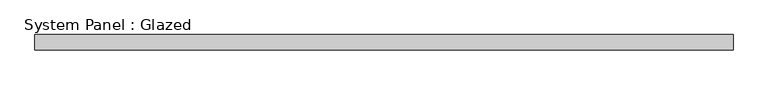
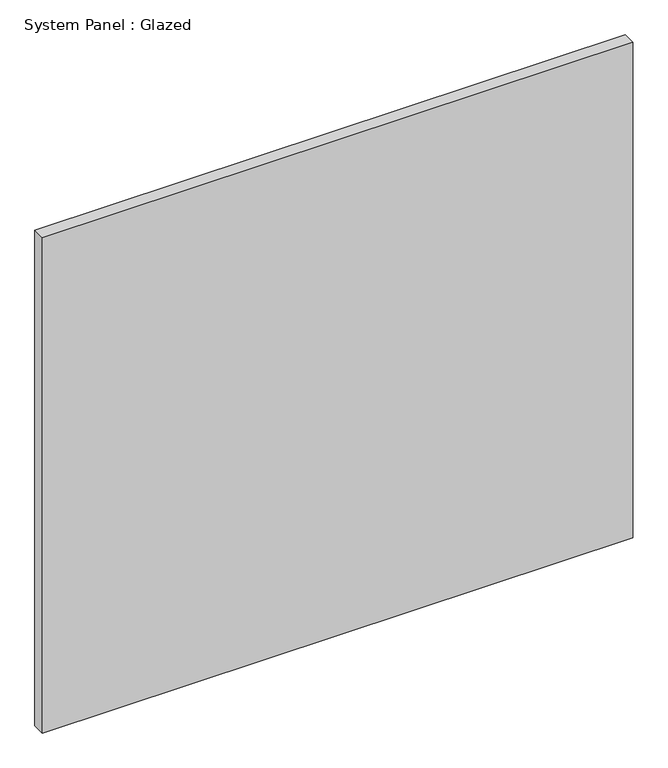
"""IFC4 building model written with IfcOpenShell, lengths in millimetres: plate geometry, System Panel : Glazed."""

from ifc_helpers import new_model, si_unit, origin, origin_with_axes, place, context, project, spatial, polyline, outline, extrude, source, transform, mapped, element, save


def system_panel_glazed_eb972c8e(model_context):
    return source(origin(), model_context, "Body", "SweptSolid", [
        extrude(outline(polyline([(581.0249999, 19.05), (-581.0249999, 19.05), (-581.0249999, 44.45), (581.0249999, 44.45), (581.0249999, 19.05)])), origin_with_axes(), (0.0, 0.0, 1.0), 1030.2424454),
    ])


if __name__ == "__main__":
    model = new_model("IFC4")
    model_context = context("Model", 3, world=origin())
    ifc_project = project(units=[si_unit("LENGTHUNIT", "METRE", prefix="MILLI")], contexts=[model_context])
    site = spatial("IfcSite", under=ifc_project)
    building = spatial("IfcBuilding", under=site)
    placement = place(None, origin())
    system_panel_glazed_shape = system_panel_glazed_eb972c8e(model_context)
    element("IfcPlate", 1, ObjectType="System Panel : Glazed", at=placement, inside=building, context=model_context, shape_type="MappedRepresentation", body=[
        mapped(system_panel_glazed_shape, transform((0.0, 0.0, 0.0), x_axis=(1.0, 0.0, 0.0), y_axis=(0.0, 1.0, 0.0), z_axis=(0.0, 0.0, 1.0))),
    ])
    save(model, "model.ifc")

# Revit data of these elements
# Type "System Panel : Glazed"
#   Construction Type Id = "GSP4R"
#   Analytic Construction = "1/8 in Pilkington single glazing"
#   Visual Light Transmittance = 0.9
#   Solar Heat Gain Coefficient = 0.86
#   Heat Transfer Coefficient (U) = 1.18115 BTU/(h·ft²·°F)
#   Define Thermal Properties by = 1
# Element 1 (IfcPlate, "System Panel : Glazed")
#   Materials on its faces: "Glass"
# Materials
#   "Glass": class "Glass", colour RGB 0 128 192, transparency 0.75, Description = "Soda Lime Glass", Cost = 0
